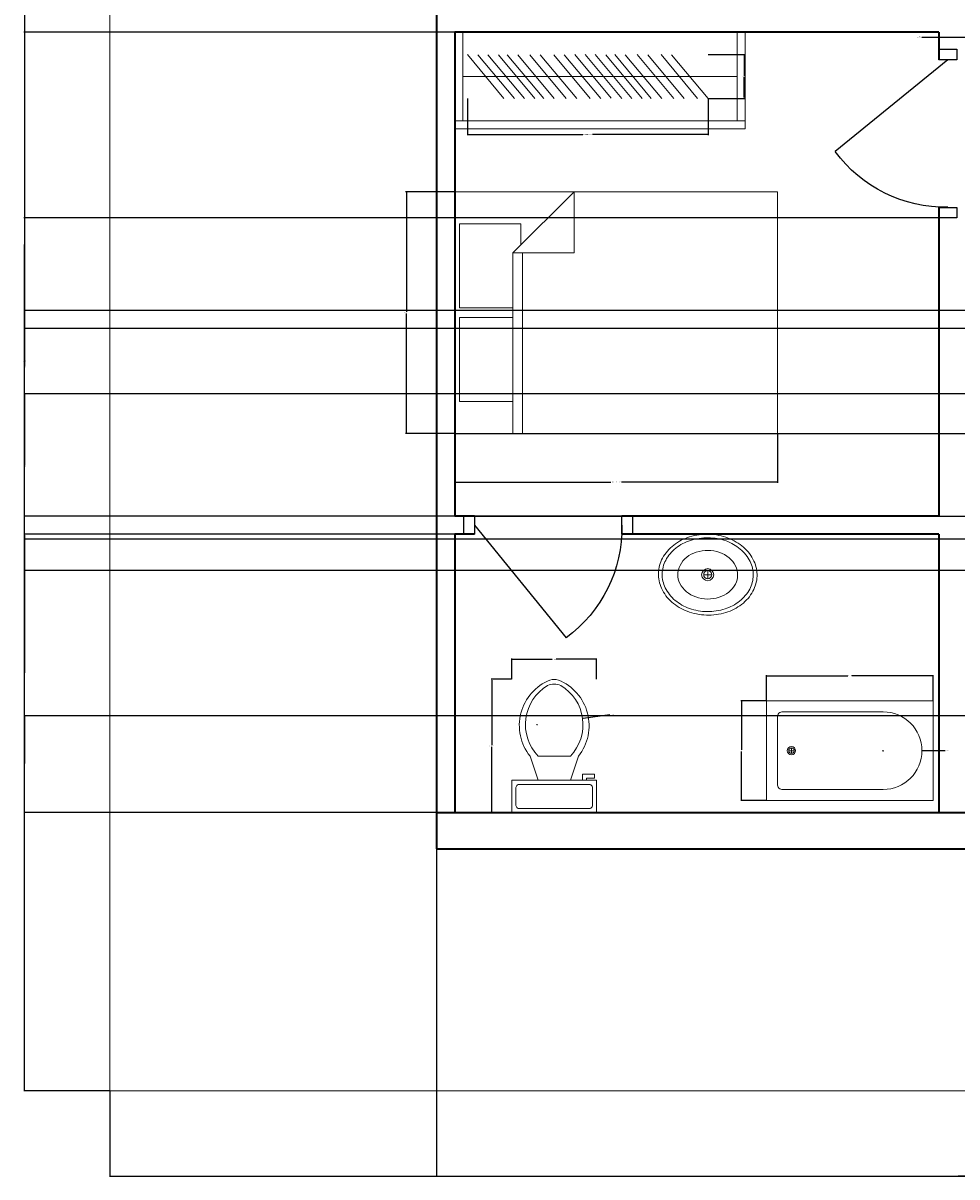
# Model space of a CAD drawing. Units: inches. Extents: x 109 to 572, y -157 to 568.
# Tile 1 of 5: x 109 to 341, y 105 to 391. Entities that reach past the tile are written whole.
import ezdxf

# ---------------------------------------------------------------- set-up
doc = ezdxf.new("R2010")
doc.units = ezdxf.units.IN
for name, color, linetype, lineweight in [('A-ANNO-DIMS', 2, 'Continuous', 18), ('A-FLOR-CASE', 32, 'Continuous', 18), ('A-FLOR-FIXT', 4, 'Continuous', 18), ('A-WALL', 7, 'Continuous', 35), ('C-PROP', 8, 'Continuous', 18), ('DOOR.', 240, 'Continuous', 25), ('FURNUTURE', 50, 'Continuous', 18)]:
    doc.layers.add(name, color=color, linetype=linetype, lineweight=lineweight)
doc.styles.get("Standard").update_dxf_attribs({"font": 'arial.ttf'})
doc.dimstyles.get("Standard").update_dxf_attribs({"dimtxt": 0.18, "dimasz": 0.18, "dimexe": 0.18, "dimexo": 0.0625, "dimgap": 0.09, "dimtad": 0, "dimtih": 1, "dimtoh": 1, "dimdec": 4, "dimzin": 0, "dimdsep": 46, "dimtxsty": 'Standard', "dimcen": 0.09, "dimadec": 0, "dimazin": 0, "dimtfac": 1, "dimtdec": 4, "dimtofl": 0, "dimtmove": 0, "dimatfit": 3, "dimfxl": 1, "dimtolj": 1, "dimtzin": 0, "dimarcsym": 0})

# ---------------------------------------------------------------- blocks, each defined once
blk = doc.blocks.new('Sink - Oval top')
for p, q in [((-1, 0), (1, 0)), ((0, 1), (0, -1))]:
    blk.add_line(p, q)
for points in [[(-12.23, 0.39, 0.117634), (-11.46, -3.36, 0.104469), (-8.88, -6.8, 0.090016), (-5.08, -9.07, 0.08192), (-0.32, -10.02, 0.08192), (4.49, -9.38, 0.090016), (8.42, -7.36, 0.104469), (11.22, -4.09, 0.117634), (12.23, -0.39, 0.117634), (11.46, 3.36, 0.104469), (8.88, 6.8, 0.090016), (5.08, 9.07, 0.08192), (0.32, 10.02, 0.08192), (-4.49, 9.38, 0.090016), (-8.42, 7.36, 0.104469), (-11.22, 4.09, 0.117634)], [(-11.29, 0.16, 0.118622), (-10.52, -3.25, 0.104678), (-8.07, -6.36, 0.089562), (-4.54, -8.37, 0.081185), (-0.13, -9.15, 0.081185), (4.3, -8.49, 0.089562), (7.89, -6.58, 0.104678), (10.42, -3.55, 0.118622), (11.29, -0.16, 0.118622), (10.52, 3.25, 0.104678), (8.07, 6.36, 0.089562), (4.54, 8.37, 0.081185), (0.13, 9.15, 0.081185), (-4.3, 8.49, 0.089562), (-7.89, 6.58, 0.104678), (-10.42, 3.55, 0.118622)], [(-7.42, 0.08, 0.118283), (-6.91, -2.17, 0.104607), (-5.29, -4.21, 0.089718), (-2.97, -5.53, 0.081436), (-0.07, -6.04, 0.081436), (2.84, -5.59, 0.089718), (5.2, -4.33, 0.104607), (6.86, -2.32, 0.118283), (7.42, -0.08, 0.118283), (6.91, 2.17, 0.104607), (5.29, 4.21, 0.089718), (2.97, 5.53, 0.081436), (0.07, 6.04, 0.081436), (-2.84, 5.59, 0.089718), (-5.2, 4.33, 0.104607), (-6.86, 2.32, 0.118283)]]:
    blk.add_lwpolyline(points, format="xyb", close=True)
for radius in [1.5, 1]:
    blk.add_circle((0, 0), radius)
blk = doc.blocks.new('Bath Tub - 26 x 60 in.')
for p, q in [((8, -18), (10, -18)), ((9, -17), (9, -19))]:
    blk.add_line(p, q)
blk.add_lwpolyline([(0, -36), (0, 0), (60, 0), (60, -36)], close=True)
for points in [[(6, -4), (42, -4)], [(4, -30), (4, -6)], [(42, -32), (6, -32)]]:
    blk.add_lwpolyline(points)
for radius in [1.5, 1]:
    blk.add_circle((9, -18), radius)
for centre, radius, start, end in [((5.75, -5.75), 1.77, 81.8699, 188.1301), ((42, -18), 14, 270, 90), ((5.75, -30.25), 1.77, 171.8699, 278.1301)]:
    blk.add_arc(centre, radius, start, end)
blk = doc.blocks.new('Bed - Queen')
for p, q in [((0, -80.00003), (0, 0)), ((0, 0), (59.99999, 0)), ((59.99999, 0), (59.99999, -80.00003)), ((7.99999, -1.2), (28.79998, -1.2)), ((7.99999, -14.4), (7.99999, -1.2)), ((28.79998, -1.2), (28.79998, -14.4)), ((31.19999, -1.2), (51.99999, -1.2)), ((31.19999, -14.4), (31.19999, -1.2)), ((51.99999, -1.2), (51.99999, -16.4)), ((0, -14.4), (44.8, -14.4)), ((44.8, -16.8), (0, -16.8)), ((59.99999, -29.6), (44.8, -14.4)), ((44.8, -14.4), (44.8, -29.6)), ((51.99999, -16.4), (46.79936, -16.4)), ((44.8, -29.6), (59.99999, -29.6)), ((59.99999, -80.00003), (0, -80.00003))]:
    blk.add_line(p, q)
blk = doc.blocks.new('Toilet - top')
for p, q in [((9.5, -6), (9.5, -2)), ((-10, -8.5), (-8, -8.5)), ((-10, -9.5), (-10, -8.5)), ((-8, -8.5), (-8, -8)), ((-7, -8), (-7, -9.5)), ((-4, -8), (-6, -14)), ((4, -8), (6, -14)), ((-7, -9.5), (-10, -9.5)), ((4, -14), (-4, -14))]:
    blk.add_line(p, q)
blk.add_lwpolyline([(10.5, -8), (10.5, 0), (-10.5, 0), (-10.5, -8)], close=True)
for points in [[(-9.5, -2), (-9.5, -6)], [(8.5, -1), (-8.5, -1)], [(-8.5, -7), (8.5, -7)]]:
    blk.add_lwpolyline(points)
for centre, radius, start, end in [((-8.62, -1.88), 0.884, 81.8699, 188.1301), ((8.62, -1.88), 0.884, 351.8699, 98.1301), ((-8.62, -6.12), 0.884, 171.8699, 278.1301), ((8.62, -6.12), 0.884, 261.8699, 8.1301), ((3.52, -21.58), 12.17, 141.4691, 247.9714), ((4.2, -21.82), 11.33, 136.3677, 238.9468), ((-3.52, -21.58), 12.17, 292.0284, 38.5307), ((-4.2, -21.82), 11.33, 301.053, 43.6321), ((0, -27.88), 4, 245.7318, 294.2682), ((0, -29), 4, 254.8605, 285.1395)]:
    blk.add_arc(centre, radius, start, end)
blk = doc.blocks.new('DOOR-SINGLE-36IN-JAMB')
blk.add_line((0, 0), (-27.91, 22.73))
for points in [[(-2.25, 36.57), (2.25, 36.57), (2.25, 39.21), (-2.25, 39.21)], [(-2.25, -2.64), (2.25, -2.64), (2.25, 0), (-2.25, 0)]]:
    blk.add_lwpolyline(points, close=True)
blk.add_arc((-0.58, 2.67), 33.9, 89.0125, 143.7179)
blk = doc.blocks.new('CLOSET-FRAME-RAIL-72IN')
for p, q in [((0, 0), (0, 24)), ((0, 24), (72, 24)), ((72, 24), (72, 0)), ((0, 22), (72, 22)), ((2, 0), (2, 22)), ((70, 22), (70, 0)), ((2, 11), (70, 11))]:
    blk.add_line(p, q)
blk = doc.blocks.new('CLOSET-HANGERS')
for p, q in [((0, 0), (-9.05, 10.83)), ((2.61, -0.01), (-6.44, 10.82)), ((5.08, -0.01), (-3.97, 10.82)), ((7.69, -0.01), (-1.36, 10.82)), ((9.9, -0.01), (0.85, 10.82)), ((12.51, -0.01), (3.46, 10.82)), ((15.48, -0.01), (6.43, 10.82)), ((18.09, -0.01), (9.04, 10.82)), ((21.4, -0.01), (12.35, 10.82)), ((24.01, -0.01), (14.96, 10.82)), ((26.62, 0.01), (17.57, 10.84)), ((29.23, 0), (20.18, 10.83)), ((31.7, 0), (22.65, 10.83)), ((34.31, -0.01), (25.26, 10.82)), ((36.52, 0), (27.47, 10.83)), ((39.13, -0.01), (30.08, 10.82)), ((42.1, 0), (33.05, 10.83)), ((44.71, -0.01), (35.66, 10.82)), ((48.01, 0), (38.97, 10.83)), ((50.63, -0.01), (41.58, 10.82))]:
    blk.add_line(p, q)
blk = doc.blocks.new('*D17')
at = {"layer": 'A-ANNO-DIMS', "color": 0, "lineweight": -2, "transparency": 16777216}
for p, q in [((216.02, 289.43), (216.02, 277.31)), ((296.02, 289.43), (296.02, 277.31)), ((216.2, 277.49), (254.72, 277.49)), ((295.84, 277.49), (257.32, 277.49))]:
    blk.add_line(p, q, dxfattribs=at)
at = {"layer": 'A-ANNO-DIMS', "color": 0, "transparency": 16777216}
for points in [[(216.2, 277.52), (216.2, 277.46), (216.02, 277.49)], [(295.84, 277.52), (295.84, 277.46), (296.02, 277.49)]]:
    blk.add_solid(points, dxfattribs=at)
at = {"layer": 'Defpoints', "color": 0, "transparency": 16777216}
for p in [(216.02, 289.49), (296.02, 289.49), (216.02, 277.49)]:
    blk.add_point(p, dxfattribs=at)
at = {"layer": 'A-ANNO-DIMS', "color": 0, "transparency": 16777216, "insert": (256.02, 277.49), "char_height": 0.18, "attachment_point": 5}
blk.add_mtext('\\A1;QUEEN BED 80 TYP.', dxfattribs=at)
blk = doc.blocks.new('*D18')
at = {"layer": 'A-ANNO-DIMS', "color": 0, "lineweight": -2, "transparency": 16777216}
for p, q in [((215.96, 349.49), (203.84, 349.49)), ((204.02, 349.31), (204.02, 319.67)), ((204.02, 289.67), (204.02, 319.31)), ((215.96, 289.49), (203.84, 289.49))]:
    blk.add_line(p, q, dxfattribs=at)
at = {"layer": 'A-ANNO-DIMS', "color": 0, "transparency": 16777216}
for points in [[(203.99, 349.31), (204.05, 349.31), (204.02, 349.49)], [(203.99, 289.67), (204.05, 289.67), (204.02, 289.49)]]:
    blk.add_solid(points, dxfattribs=at)
at = {"layer": 'Defpoints', "color": 0, "transparency": 16777216}
for p in [(204.02, 349.49), (216.02, 349.49), (216.02, 289.49)]:
    blk.add_point(p, dxfattribs=at)
at = {"layer": 'A-ANNO-DIMS', "color": 0, "transparency": 16777216, "insert": (204.02, 319.49), "char_height": 0.18, "attachment_point": 5}
blk.add_mtext('\\A1;60 TYP.', dxfattribs=at)
blk = doc.blocks.new('*D23')
at = {"layer": 'A-ANNO-DIMS', "color": 0, "lineweight": -2, "transparency": 16777216}
for p, q in [((230.11, 228.59), (225.04, 228.59)), ((225.22, 228.41), (225.22, 212.25)), ((225.22, 195.72), (225.22, 211.88)), ((230.11, 195.54), (225.04, 195.54))]:
    blk.add_line(p, q, dxfattribs=at)
at = {"layer": 'A-ANNO-DIMS', "color": 0, "transparency": 16777216}
for points in [[(225.19, 228.41), (225.25, 228.41), (225.22, 228.59)], [(225.19, 195.72), (225.25, 195.72), (225.22, 195.54)]]:
    blk.add_solid(points, dxfattribs=at)
at = {"layer": 'Defpoints', "color": 0, "transparency": 16777216}
for p in [(230.18, 228.59), (225.22, 195.54), (230.18, 195.54)]:
    blk.add_point(p, dxfattribs=at)
at = {"layer": 'A-ANNO-DIMS', "color": 0, "transparency": 16777216, "insert": (225.22, 212.06), "char_height": 0.18, "attachment_point": 5}
blk.add_mtext('\\A1;WC 33 TYP.', dxfattribs=at)
blk = doc.blocks.new('*D24')
at = {"layer": 'A-ANNO-DIMS', "color": 0, "lineweight": -2, "transparency": 16777216}
for p, q in [((230.18, 228.65), (230.18, 233.72)), ((230.36, 233.54), (240.15, 233.54)), ((251, 233.54), (241.2, 233.54)), ((251.18, 228.65), (251.18, 233.72))]:
    blk.add_line(p, q, dxfattribs=at)
at = {"layer": 'A-ANNO-DIMS', "color": 0, "transparency": 16777216}
for points in [[(230.36, 233.57), (230.36, 233.51), (230.18, 233.54)], [(251, 233.57), (251, 233.51), (251.18, 233.54)]]:
    blk.add_solid(points, dxfattribs=at)
at = {"layer": 'Defpoints', "color": 0, "transparency": 16777216}
for p in [(230.18, 233.54), (230.18, 228.59), (251.18, 228.59)]:
    blk.add_point(p, dxfattribs=at)
at = {"layer": 'A-ANNO-DIMS', "color": 0, "transparency": 16777216, "insert": (240.68, 233.54), "char_height": 0.18, "attachment_point": 5}
blk.add_mtext('\\A1;21 TYP.', dxfattribs=at)
blk = doc.blocks.new('*D27')
at = {"layer": 'A-ANNO-DIMS', "color": 0, "lineweight": -2, "transparency": 16777216}
for p, q in [((219.15, 372.56), (219.15, 363.49)), ((278.82, 372.56), (278.82, 363.49)), ((219.33, 363.67), (247.81, 363.67)), ((278.64, 363.67), (250.16, 363.67))]:
    blk.add_line(p, q, dxfattribs=at)
at = {"layer": 'A-ANNO-DIMS', "color": 0, "transparency": 16777216}
for points in [[(219.33, 363.7), (219.33, 363.64), (219.15, 363.67)], [(278.64, 363.7), (278.64, 363.64), (278.82, 363.67)]]:
    blk.add_solid(points, dxfattribs=at)
at = {"layer": 'Defpoints', "color": 0, "transparency": 16777216}
for p in [(219.15, 372.62), (278.82, 372.62), (278.82, 363.67)]:
    blk.add_point(p, dxfattribs=at)
at = {"layer": 'A-ANNO-DIMS', "color": 0, "transparency": 16777216, "insert": (248.99, 363.67), "char_height": 0.18, "attachment_point": 5}
blk.add_mtext('\\A1;HANGERS 60 TYP.', dxfattribs=at)
blk = doc.blocks.new('*D28')
at = {"layer": 'A-ANNO-DIMS', "color": 0, "lineweight": -2, "transparency": 16777216}
for p, q in [((278.88, 383.47), (287.95, 383.47)), ((287.77, 383.29), (287.77, 378.22)), ((287.77, 372.8), (287.77, 377.86)), ((278.88, 372.62), (287.95, 372.62))]:
    blk.add_line(p, q, dxfattribs=at)
at = {"layer": 'A-ANNO-DIMS', "color": 0, "transparency": 16777216}
for points in [[(287.74, 383.29), (287.8, 383.29), (287.77, 383.47)], [(287.74, 372.8), (287.8, 372.8), (287.77, 372.62)]]:
    blk.add_solid(points, dxfattribs=at)
at = {"layer": 'Defpoints', "color": 0, "transparency": 16777216}
for p in [(278.82, 383.47), (287.77, 383.47), (278.82, 372.62)]:
    blk.add_point(p, dxfattribs=at)
at = {"layer": 'A-ANNO-DIMS', "color": 0, "transparency": 16777216, "insert": (287.77, 378.04), "char_height": 0.18, "attachment_point": 5}
blk.add_mtext('\\A1;11 TYP.', dxfattribs=at)
blk = doc.blocks.new('*D37')
at = {"layer": 'A-ANNO-DIMS', "color": 0, "lineweight": -2, "transparency": 16777216}
for p, q in [((293.3, 223.34), (293.3, 229.65)), ((293.48, 229.47), (313.46, 229.47)), ((334.41, 229.47), (314.44, 229.47)), ((334.59, 223.34), (334.59, 229.65))]:
    blk.add_line(p, q, dxfattribs=at)
at = {"layer": 'A-ANNO-DIMS', "color": 0, "transparency": 16777216}
for points in [[(293.48, 229.5), (293.48, 229.44), (293.3, 229.47)], [(334.41, 229.5), (334.41, 229.44), (334.59, 229.47)]]:
    blk.add_solid(points, dxfattribs=at)
at = {"layer": 'Defpoints', "color": 0, "transparency": 16777216}
for p in [(334.59, 229.47), (293.3, 223.28), (334.59, 223.28)]:
    blk.add_point(p, dxfattribs=at)
at = {"layer": 'A-ANNO-DIMS', "color": 0, "transparency": 16777216, "insert": (313.95, 229.47), "char_height": 0.18, "attachment_point": 5}
blk.add_mtext('\\A1;TUB 41', dxfattribs=at)
blk = doc.blocks.new('*D38')
at = {"layer": 'A-ANNO-DIMS', "color": 0, "lineweight": -2, "transparency": 16777216}
for p, q in [((293.24, 223.28), (286.93, 223.28)), ((287.11, 223.1), (287.11, 211.07)), ((287.11, 198.69), (287.11, 210.71)), ((293.24, 198.51), (286.93, 198.51))]:
    blk.add_line(p, q, dxfattribs=at)
at = {"layer": 'A-ANNO-DIMS', "color": 0, "transparency": 16777216}
for points in [[(287.08, 223.1), (287.14, 223.1), (287.11, 223.28)], [(287.08, 198.69), (287.14, 198.69), (287.11, 198.51)]]:
    blk.add_solid(points, dxfattribs=at)
at = {"layer": 'Defpoints', "color": 0, "transparency": 16777216}
for p in [(287.11, 223.28), (293.3, 223.28), (293.3, 198.51)]:
    blk.add_point(p, dxfattribs=at)
at = {"layer": 'A-ANNO-DIMS', "color": 0, "transparency": 16777216, "insert": (287.11, 210.89), "char_height": 0.18, "attachment_point": 5}
blk.add_mtext('\\A1;25', dxfattribs=at)
blk = doc.blocks.new('*D39')
at = {"layer": 'A-ANNO-DIMS', "color": 0, "lineweight": -2, "transparency": 16777216}
for p, q in [((130.52, 126.48), (130.52, 105.21)), ((550.52, 126.48), (550.52, 105.21)), ((130.7, 105.39), (340.23, 105.39)), ((550.34, 105.39), (340.81, 105.39))]:
    blk.add_line(p, q, dxfattribs=at)
at = {"layer": 'A-ANNO-DIMS', "color": 0, "transparency": 16777216}
for points in [[(130.7, 105.42), (130.7, 105.36), (130.52, 105.39)], [(550.34, 105.42), (550.34, 105.36), (550.52, 105.39)]]:
    blk.add_solid(points, dxfattribs=at)
at = {"layer": 'Defpoints', "color": 0, "transparency": 16777216}
for p in [(130.52, 126.54), (550.52, 126.54), (550.52, 105.39)]:
    blk.add_point(p, dxfattribs=at)
at = {"layer": 'A-ANNO-DIMS', "color": 0, "transparency": 16777216, "insert": (340.52, 105.39), "char_height": 0.18, "attachment_point": 5}
blk.add_mtext('\\A1;420', dxfattribs=at)
blk = doc.blocks.new('*D40')
at = {"layer": 'A-ANNO-DIMS', "color": 0, "lineweight": -2, "transparency": 16777216}
for p, q in [((130.46, 546.54), (109.19, 546.54)), ((109.37, 546.36), (109.37, 336.72)), ((109.37, 126.72), (109.37, 336.36)), ((130.46, 126.54), (109.19, 126.54))]:
    blk.add_line(p, q, dxfattribs=at)
at = {"layer": 'A-ANNO-DIMS', "color": 0, "transparency": 16777216}
for points in [[(109.34, 546.36), (109.4, 546.36), (109.37, 546.54)], [(109.34, 126.72), (109.4, 126.72), (109.37, 126.54)]]:
    blk.add_solid(points, dxfattribs=at)
at = {"layer": 'Defpoints', "color": 0, "transparency": 16777216}
for p in [(109.37, 546.54), (130.52, 546.54), (130.52, 126.54)]:
    blk.add_point(p, dxfattribs=at)
at = {"layer": 'A-ANNO-DIMS', "color": 0, "transparency": 16777216, "insert": (109.37, 336.54), "char_height": 0.18, "attachment_point": 5}
blk.add_mtext('\\A1;420', dxfattribs=at)
blk = doc.blocks.new('*D43')
at = {"layer": 'A-ANNO-DIMS', "color": 0, "lineweight": -2, "transparency": 16777216}
for p, q in [((211.52, 186.48), (211.52, 105.21)), ((526.52, 186.48), (526.52, 105.21)), ((211.7, 105.39), (368.73, 105.39)), ((526.34, 105.39), (369.31, 105.39))]:
    blk.add_line(p, q, dxfattribs=at)
at = {"layer": 'A-ANNO-DIMS', "color": 0, "transparency": 16777216}
for points in [[(211.7, 105.42), (211.7, 105.36), (211.52, 105.39)], [(526.34, 105.42), (526.34, 105.36), (526.52, 105.39)]]:
    blk.add_solid(points, dxfattribs=at)
at = {"layer": 'Defpoints', "color": 0, "transparency": 16777216}
for p in [(211.52, 186.54), (526.52, 186.54), (526.52, 105.39)]:
    blk.add_point(p, dxfattribs=at)
at = {"layer": 'A-ANNO-DIMS', "color": 0, "transparency": 16777216, "insert": (369.02, 105.39), "char_height": 0.18, "attachment_point": 5}
blk.add_mtext('\\A1;315', dxfattribs=at)
blk = doc.blocks.new('*D48')
at = {"layer": 'A-ANNO-DIMS', "color": 0, "lineweight": -2, "transparency": 16777216}
for p, q in [((215.96, 264.54), (109.19, 264.54)), ((109.37, 264.36), (109.37, 230.22)), ((109.37, 195.72), (109.37, 229.86)), ((215.96, 195.54), (109.19, 195.54))]:
    blk.add_line(p, q, dxfattribs=at)
at = {"layer": 'A-ANNO-DIMS', "color": 0, "transparency": 16777216}
for points in [[(109.34, 264.36), (109.4, 264.36), (109.37, 264.54)], [(109.34, 195.72), (109.4, 195.72), (109.37, 195.54)]]:
    blk.add_solid(points, dxfattribs=at)
at = {"layer": 'Defpoints', "color": 0, "transparency": 16777216}
for p in [(109.37, 264.54), (216.02, 264.54), (216.02, 195.54)]:
    blk.add_point(p, dxfattribs=at)
at = {"layer": 'A-ANNO-DIMS', "color": 0, "transparency": 16777216, "insert": (109.37, 230.04), "char_height": 0.18, "attachment_point": 5}
blk.add_mtext('\\A1;69', dxfattribs=at)
blk = doc.blocks.new('*D49')
at = {"layer": 'A-ANNO-DIMS', "color": 0, "lineweight": -2, "transparency": 16777216}
for p, q in [((215.96, 389.04), (109.19, 389.04)), ((109.37, 388.86), (109.37, 329.22)), ((109.37, 269.22), (109.37, 328.86)), ((215.96, 269.04), (109.19, 269.04))]:
    blk.add_line(p, q, dxfattribs=at)
at = {"layer": 'A-ANNO-DIMS', "color": 0, "transparency": 16777216}
for points in [[(109.34, 388.86), (109.4, 388.86), (109.37, 389.04)], [(109.34, 269.22), (109.4, 269.22), (109.37, 269.04)]]:
    blk.add_solid(points, dxfattribs=at)
at = {"layer": 'Defpoints', "color": 0, "transparency": 16777216}
for p in [(109.37, 389.04), (216.02, 389.04), (216.02, 269.04)]:
    blk.add_point(p, dxfattribs=at)
at = {"layer": 'A-ANNO-DIMS', "color": 0, "transparency": 16777216, "insert": (109.37, 329.04), "char_height": 0.18, "attachment_point": 5}
blk.add_mtext('\\A1;120', dxfattribs=at)
blk = doc.blocks.new('*D55')
at = {"layer": 'A-ANNO-DIMS', "color": 0, "lineweight": -2, "transparency": 16777216}
for p, q in [((493.46, 299.4), (109.19, 299.4)), ((109.37, 299.22), (109.37, 281.56)), ((109.37, 263.53), (109.37, 281.2)), ((493.46, 263.35), (109.19, 263.35))]:
    blk.add_line(p, q, dxfattribs=at)
at = {"layer": 'A-ANNO-DIMS', "color": 0, "transparency": 16777216}
for points in [[(109.34, 299.22), (109.4, 299.22), (109.37, 299.4)], [(109.34, 263.53), (109.4, 263.53), (109.37, 263.35)]]:
    blk.add_solid(points, dxfattribs=at)
at = {"layer": 'Defpoints', "color": 0, "transparency": 16777216}
for p in [(109.37, 299.4), (493.52, 299.4), (493.52, 263.35)]:
    blk.add_point(p, dxfattribs=at)
at = {"layer": 'A-ANNO-DIMS', "color": 0, "transparency": 16777216, "insert": (109.37, 281.38), "char_height": 0.18, "attachment_point": 5}
blk.add_mtext('\\A1;36.05', dxfattribs=at)
blk = doc.blocks.new('*D56')
at = {"layer": 'A-ANNO-DIMS', "color": 0, "lineweight": -2, "transparency": 16777216}
for p, q in [((493.46, 255.54), (109.19, 255.54)), ((109.37, 255.36), (109.37, 237.72)), ((109.37, 219.72), (109.37, 237.36)), ((493.46, 219.54), (109.19, 219.54))]:
    blk.add_line(p, q, dxfattribs=at)
at = {"layer": 'A-ANNO-DIMS', "color": 0, "transparency": 16777216}
for points in [[(109.34, 255.36), (109.4, 255.36), (109.37, 255.54)], [(109.34, 219.72), (109.4, 219.72), (109.37, 219.54)]]:
    blk.add_solid(points, dxfattribs=at)
at = {"layer": 'Defpoints', "color": 0, "transparency": 16777216}
for p in [(493.52, 255.54), (109.37, 219.54), (493.52, 219.54)]:
    blk.add_point(p, dxfattribs=at)
at = {"layer": 'A-ANNO-DIMS', "color": 0, "transparency": 16777216, "insert": (109.37, 237.54), "char_height": 0.18, "attachment_point": 5}
blk.add_mtext('\\A1;36', dxfattribs=at)
blk = doc.blocks.new('*D58')
at = {"layer": 'A-ANNO-DIMS', "color": 0, "lineweight": -2, "transparency": 16777216}
for p, q in [((335.96, 342.97), (109.19, 342.97)), ((109.37, 342.79), (109.37, 306.19)), ((109.37, 269.22), (109.37, 305.82)), ((335.96, 269.04), (109.19, 269.04))]:
    blk.add_line(p, q, dxfattribs=at)
at = {"layer": 'A-ANNO-DIMS', "color": 0, "transparency": 16777216}
for points in [[(109.34, 342.79), (109.4, 342.79), (109.37, 342.97)], [(109.34, 269.22), (109.4, 269.22), (109.37, 269.04)]]:
    blk.add_solid(points, dxfattribs=at)
at = {"layer": 'Defpoints', "color": 0, "transparency": 16777216}
for p in [(109.37, 342.97), (336.02, 342.97), (336.02, 269.04)]:
    blk.add_point(p, dxfattribs=at)
at = {"layer": 'A-ANNO-DIMS', "color": 0, "transparency": 16777216, "insert": (109.37, 306), "char_height": 0.18, "attachment_point": 5}
blk.add_mtext('\\A1;73.93', dxfattribs=at)
blk = doc.blocks.new('*D63')
at = {"layer": 'A-ANNO-DIMS', "color": 0, "lineweight": -2, "transparency": 16777216}
for p, q in [((457.46, 320.04), (109.19, 320.04)), ((109.37, 319.86), (109.37, 317.97)), ((109.37, 315.72), (109.37, 317.61)), ((457.46, 315.54), (109.19, 315.54))]:
    blk.add_line(p, q, dxfattribs=at)
at = {"layer": 'A-ANNO-DIMS', "color": 0, "transparency": 16777216}
for points in [[(109.34, 319.86), (109.4, 319.86), (109.37, 320.04)], [(109.34, 315.72), (109.4, 315.72), (109.37, 315.54)]]:
    blk.add_solid(points, dxfattribs=at)
at = {"layer": 'Defpoints', "color": 0, "transparency": 16777216}
for p in [(109.37, 320.04), (457.52, 320.04), (457.52, 315.54)]:
    blk.add_point(p, dxfattribs=at)
at = {"layer": 'A-ANNO-DIMS', "color": 0, "transparency": 16777216, "insert": (109.37, 317.79), "char_height": 0.18, "attachment_point": 5}
blk.add_mtext('\\A1;4.5', dxfattribs=at)
blk = doc.blocks.new('*D67')
at = {"layer": 'A-ANNO-DIMS', "color": 0, "lineweight": -2, "transparency": 16777216}
for p, q in [((457.46, 219.54), (109.19, 219.54)), ((109.37, 219.36), (109.37, 207.72)), ((109.37, 195.72), (109.37, 207.36)), ((457.46, 195.54), (109.19, 195.54))]:
    blk.add_line(p, q, dxfattribs=at)
at = {"layer": 'A-ANNO-DIMS', "color": 0, "transparency": 16777216}
for points in [[(109.34, 219.36), (109.4, 219.36), (109.37, 219.54)], [(109.34, 195.72), (109.4, 195.72), (109.37, 195.54)]]:
    blk.add_solid(points, dxfattribs=at)
at = {"layer": 'Defpoints', "color": 0, "transparency": 16777216}
for p in [(457.52, 219.54), (109.37, 195.54), (457.52, 195.54)]:
    blk.add_point(p, dxfattribs=at)
at = {"layer": 'A-ANNO-DIMS', "color": 0, "transparency": 16777216, "insert": (109.37, 207.54), "char_height": 0.18, "attachment_point": 5}
blk.add_mtext('\\A1;24', dxfattribs=at)
blk = doc.blocks.new('*D69')
at = {"layer": 'A-ANNO-DIMS', "color": 0, "lineweight": -2, "transparency": 16777216}
for p, q in [((216.08, 289.49), (571.85, 289.49)), ((571.67, 289.31), (571.67, 279.45)), ((571.67, 269.22), (571.67, 279.08)), ((216.08, 269.04), (571.85, 269.04))]:
    blk.add_line(p, q, dxfattribs=at)
at = {"layer": 'A-ANNO-DIMS', "color": 0, "transparency": 16777216}
for points in [[(571.64, 289.31), (571.7, 289.31), (571.67, 289.49)], [(571.64, 269.22), (571.7, 269.22), (571.67, 269.04)]]:
    blk.add_solid(points, dxfattribs=at)
at = {"layer": 'Defpoints', "color": 0, "transparency": 16777216}
for p in [(216.02, 289.49), (571.67, 289.49), (216.02, 269.04)]:
    blk.add_point(p, dxfattribs=at)
at = {"layer": 'A-ANNO-DIMS', "color": 0, "transparency": 16777216, "insert": (571.67, 279.26), "char_height": 0.18, "attachment_point": 5}
blk.add_mtext('\\A1;20.45', dxfattribs=at)
blk = doc.blocks.new('*D70')
at = {"layer": 'A-ANNO-DIMS', "color": 0, "lineweight": -2, "transparency": 16777216}
for p, q in [((517.46, 315.54), (109.19, 315.54)), ((109.37, 315.36), (109.37, 307.65)), ((109.37, 299.58), (109.37, 307.29)), ((517.46, 299.4), (109.19, 299.4))]:
    blk.add_line(p, q, dxfattribs=at)
at = {"layer": 'A-ANNO-DIMS', "color": 0, "transparency": 16777216}
for points in [[(109.34, 315.36), (109.4, 315.36), (109.37, 315.54)], [(109.34, 299.58), (109.4, 299.58), (109.37, 299.4)]]:
    blk.add_solid(points, dxfattribs=at)
at = {"layer": 'Defpoints', "color": 0, "transparency": 16777216}
for p in [(517.52, 315.54), (109.37, 299.4), (517.52, 299.4)]:
    blk.add_point(p, dxfattribs=at)
at = {"layer": 'A-ANNO-DIMS', "color": 0, "transparency": 16777216, "insert": (109.37, 307.47), "char_height": 0.18, "attachment_point": 5}
blk.add_mtext('\\A1;16.136', dxfattribs=at)
blk = doc.blocks.new('*D74')
at = {"layer": 'A-ANNO-DIMS', "color": 0, "lineweight": -2, "transparency": 16777216}
for p, q in [((331.8, 387.8), (374.88, 387.8)), ((447.07, 387.8), (447.25, 387.8)), ((447.16, 387.71), (447.16, 387.89))]:
    blk.add_line(p, q, dxfattribs=at)
at = {"layer": 'A-ANNO-DIMS', "color": 0, "transparency": 16777216}
blk.add_solid([(374.88, 387.83), (374.88, 387.77), (375.06, 387.8)], dxfattribs=at)
at = {"layer": 'Defpoints', "color": 0, "transparency": 16777216}
for p in [(375.06, 387.8), (447.16, 387.8)]:
    blk.add_point(p, dxfattribs=at)
at = {"layer": 'A-ANNO-DIMS', "color": 0, "transparency": 16777216, "insert": (331.21, 387.8), "char_height": 0.18, "attachment_point": 5}
blk.add_mtext('\\A1;2X R72.1', dxfattribs=at)
blk = doc.blocks.new('*D76')
at = {"layer": 'A-ANNO-DIMS', "color": 0, "lineweight": -2, "transparency": 16777216}
for p, q in [((236.48, 217.27), (236.48, 217.45)), ((254.44, 219.77), (247.88, 218.89)), ((236.39, 217.36), (236.57, 217.36))]:
    blk.add_line(p, q, dxfattribs=at)
at = {"layer": 'A-ANNO-DIMS', "color": 0, "transparency": 16777216}
blk.add_solid([(247.88, 218.92), (247.89, 218.86), (247.7, 218.87)], dxfattribs=at)
at = {"layer": 'Defpoints', "color": 0, "transparency": 16777216}
for p in [(247.7, 218.87), (236.48, 217.36)]:
    blk.add_point(p, dxfattribs=at)
at = {"layer": 'A-ANNO-DIMS', "color": 0, "transparency": 16777216, "insert": (255.12, 219.77), "char_height": 0.18, "attachment_point": 5}
blk.add_mtext('\\A1;4X R11.33', dxfattribs=at)
blk = doc.blocks.new('*D78')
at = {"layer": 'A-ANNO-DIMS', "color": 0, "lineweight": -2, "transparency": 16777216}
for p, q in [((322.11, 210.89), (322.29, 210.89)), ((322.2, 210.8), (322.2, 210.98)), ((337.62, 210.89), (332.02, 210.89))]:
    blk.add_line(p, q, dxfattribs=at)
at = {"layer": 'A-ANNO-DIMS', "color": 0, "transparency": 16777216}
blk.add_solid([(332.02, 210.92), (332.02, 210.86), (331.84, 210.89)], dxfattribs=at)
at = {"layer": 'Defpoints', "color": 0, "transparency": 16777216}
for p in [(322.2, 210.89), (331.84, 210.89)]:
    blk.add_point(p, dxfattribs=at)
at = {"layer": 'A-ANNO-DIMS', "color": 0, "transparency": 16777216, "insert": (338.1, 210.89), "char_height": 0.18, "attachment_point": 5}
blk.add_mtext('\\A1;R9.634', dxfattribs=at)

msp = doc.modelspace()

# ---------------------------------------------------------------- linework, layer by layer
at = {"layer": 'A-WALL'}
for p, q in [((211.5195, 513.5398), (211.5195, 195.5398)), ((336.0195, 389.0398), (216.0195, 389.0398)), ((216.0195, 389.0398), (216.0195, 269.0398)), ((336.0195, 389.0398), (336.0195, 382.1753)), ((336.0195, 345.6414), (336.0195, 269.0398)), ((220.8949, 269.0398), (216.0195, 269.0398)), ((336.0195, 269.0398), (257.4647, 269.0398)), ((216.0195, 264.5398), (216.0195, 195.5398)), ((220.8949, 264.5398), (216.0195, 264.5398)), ((336.0195, 264.5398), (257.4288, 264.5398)), ((336.0195, 264.5398), (336.0195, 195.5398)), ((211.5195, 195.5398), (517.5195, 195.5398)), ((211.5195, 195.5398), (211.5195, 186.5398)), ((211.5195, 186.5398), (526.5195, 186.5398))]:
    msp.add_line(p, q, dxfattribs=at)
at = {"layer": 'C-PROP'}
for p, q in [((130.5195, 546.5398), (130.5195, 126.5398)), ((130.5195, 126.5398), (550.5195, 126.5398))]:
    msp.add_line(p, q, dxfattribs=at)

# ---------------------------------------------------------------- block references
at = {"layer": 'A-FLOR-CASE', "rotation": 180}
msp.add_blockref('CLOSET-FRAME-RAIL-72IN', (288.0195, 389.0398), dxfattribs=at)
at = {"layer": 'A-FLOR-CASE'}
msp.add_blockref('CLOSET-HANGERS', (228.1956, 372.6308), dxfattribs=at)
at = {"layer": 'A-FLOR-FIXT'}
msp.add_blockref('Sink - Oval top', (278.7316, 254.5239), dxfattribs=at)
at = {"layer": 'A-FLOR-FIXT', "rotation": 180}
msp.add_blockref('Toilet - top', (240.6752, 195.5398), dxfattribs=at)
at = {"layer": 'A-FLOR-FIXT', "xscale": 0.6881205280154126, "yscale": 0.6881205280154126, "zscale": 0.6881205280154126}
msp.add_blockref('Bath Tub - 26 x 60 in.', (293.3019, 223.2784), dxfattribs=at)
at = {"layer": 'DOOR.', "extrusion": (0, 0, -1), "zscale": -1}
for p, rotation in [((-338.2695, 382.1753), 180), ((-220.8949, 266.7898), 89.99999999999979)]:
    msp.add_blockref('DOOR-SINGLE-36IN-JAMB', p, dxfattribs=dict(at, rotation=rotation))
at = {"layer": 'FURNUTURE', "rotation": 90}
msp.add_blockref('Bed - Queen', (216.0195, 289.4894), dxfattribs=at)

# ---------------------------------------------------------------- dimensions: what is measured, and where the dimension line sits
at = {"layer": 'A-ANNO-DIMS'}
for base, p1, p2, override, picture, middle in [((109.3695, 546.5398), (130.5195, 126.5398), (130.5195, 546.5398), {"dimdec": 0, "dimlfac": 1, "dimrnd": 0, "dimzin": 0, "dimdsep": 46, "dimlunit": 2}, '*D40', (109.3695, 336.5398)), ((109.3695, 389.0398), (216.0195, 269.0398), (216.0195, 389.0398), {"dimdec": 0, "dimlfac": 1, "dimrnd": 0, "dimzin": 0, "dimdsep": 46, "dimlunit": 2}, '*D49', (109.3695, 329.0398)), ((109.3695, 342.9664), (336.0195, 269.0398), (336.0195, 342.9664), {"dimdec": 2, "dimlfac": 1, "dimrnd": 0, "dimzin": 0, "dimdsep": 46, "dimlunit": 2}, '*D58', (109.3695, 306.0031)), ((109.3695, 320.0398), (457.5195, 315.5398), (457.5195, 320.0398), {"dimdec": 1, "dimlfac": 1, "dimrnd": 0, "dimzin": 0, "dimdsep": 46, "dimlunit": 2}, '*D63', (109.3695, 317.7898)), ((109.3695, 299.4036), (517.5195, 315.5398), (517.5195, 299.4036), {"dimdec": 3, "dimlfac": 1, "dimrnd": 0, "dimzin": 0, "dimdsep": 46, "dimlunit": 2}, '*D70', (109.3695, 307.4717)), ((109.3695, 299.4036), (493.5195, 263.3515), (493.5195, 299.4036), {"dimdec": 2, "dimlfac": 1, "dimrnd": 0, "dimzin": 0, "dimdsep": 46, "dimlunit": 2}, '*D55', (109.3695, 281.3775)), ((571.6695, 289.4894), (216.0195, 269.0398), (216.0195, 289.4894), {"dimdec": 2, "dimlfac": 1, "dimrnd": 0, "dimzin": 0, "dimdsep": 46, "dimlunit": 2}, '*D69', (571.6695, 279.2646)), ((109.3695, 264.5398), (216.0195, 195.5398), (216.0195, 264.5398), {"dimdec": 0, "dimlfac": 1, "dimrnd": 0, "dimzin": 0, "dimdsep": 46, "dimlunit": 2}, '*D48', (109.3695, 230.0398)), ((109.3695, 219.5398), (493.5195, 255.5398), (493.5195, 219.5398), {"dimdec": 0, "dimlfac": 1, "dimrnd": 0, "dimzin": 0, "dimdsep": 46, "dimlunit": 2}, '*D56', (109.3695, 237.5398)), ((287.1088, 223.2784), (293.3019, 198.506), (293.3019, 223.2784), {"dimdec": 0, "dimlfac": 1, "dimrnd": 0, "dimzin": 0, "dimdsep": 46, "dimlunit": 2}, '*D38', (287.1088, 210.8922)), ((109.3695, 195.5398), (457.5195, 219.5398), (457.5195, 195.5398), {"dimdec": 0, "dimlfac": 1, "dimrnd": 0, "dimzin": 0, "dimdsep": 46, "dimlunit": 2}, '*D67', (109.3695, 207.5398))]:
    dim = msp.add_linear_dim(base=base, p1=p1, p2=p2, angle=90, dimstyle='Standard', override=override, dxfattribs=at)
    dim.commit()
    dim.dimension.update_dxf_attribs({"geometry": picture, "text_midpoint": middle})
for center, mpoint, text, override, picture, middle in [((447.1629, 387.7979), (375.058, 387.798), '2X <>', {"dimdec": 1, "dimlfac": 1, "dimrnd": 0, "dimzin": 0, "dimdsep": 46, "dimlunit": 2}, '*D74', (331.7951, 387.7981)), ((236.4752, 217.3572), (247.7033, 218.867), '4X <>', {"dimdec": 2, "dimlfac": 1, "dimrnd": 0, "dimzin": 0, "dimdsep": 46, "dimlunit": 2}, '*D76', (254.4402, 219.773))]:
    dim = msp.add_radius_dim(center=center, mpoint=mpoint, text=text, dimstyle='Standard', override=override, dxfattribs=at)
    dim.commit()
    dim.dimension.update_dxf_attribs({"geometry": picture, "text_midpoint": middle, "dimtype": 164})
for base, p1, p2, angle, text, picture, middle in [((287.772, 383.466), (278.8212, 372.6193), (278.8212, 383.466), 90, '<> TYP.', '*D28', (287.772, 378.0427)), ((204.0195, 349.4894), (216.0195, 289.4894), (216.0195, 349.4894), 90, '<> TYP.', '*D18', (204.0195, 319.4894)), ((216.0195, 277.4894), (296.0196, 289.4894), (216.0195, 289.4894), 180, 'QUEEN BED <> TYP.', '*D17', (256.0196, 277.4894)), ((230.1752, 233.543), (251.1752, 228.586), (230.1752, 228.586), 180, '<> TYP.', '*D24', (240.6752, 233.543)), ((225.2182, 195.5398), (230.1752, 228.586), (230.1752, 195.5398), 270, 'WC <> TYP.', '*D23', (225.2182, 212.0629))]:
    dim = msp.add_linear_dim(base=base, p1=p1, p2=p2, angle=angle, text=text, dimstyle='Standard', override={"dimdec": 0, "dimlfac": 1, "dimrnd": 0, "dimzin": 0, "dimdsep": 46, "dimlunit": 2}, dxfattribs=at)
    dim.commit()
    dim.dimension.update_dxf_attribs({"geometry": picture, "text_midpoint": middle})
for base, p1, p2, text, picture, middle in [((278.8212, 363.6684), (219.1489, 372.6193), (278.8212, 372.6193), 'HANGERS <> TYP.', '*D27', (248.985, 363.6684)), ((334.5891, 229.4714), (293.3019, 223.2784), (334.5891, 223.2784), 'TUB <>', '*D37', (313.9455, 229.4714))]:
    dim = msp.add_linear_dim(base=base, p1=p1, p2=p2, text=text, dimstyle='Standard', override={"dimdec": 0, "dimlfac": 1, "dimrnd": 0, "dimzin": 0, "dimdsep": 46, "dimlunit": 2}, dxfattribs=at)
    dim.commit()
    dim.dimension.update_dxf_attribs({"geometry": picture, "text_midpoint": middle})
dim = msp.add_radius_dim(center=(322.203, 210.8922), mpoint=(331.8366, 210.892), dimstyle='Standard', override={"dimdec": 3, "dimlfac": 1, "dimrnd": 0, "dimzin": 0, "dimdsep": 46, "dimlunit": 2}, dxfattribs=at)
dim.commit()
dim.dimension.update_dxf_attribs({"geometry": '*D78', "text_midpoint": (337.6169, 210.8919), "dimtype": 164})
for base, p1, p2, picture, middle in [((526.5195, 105.3898), (211.5195, 186.5398), (526.5195, 186.5398), '*D43', (369.0195, 105.3898)), ((550.5195, 105.3898), (130.5195, 126.5398), (550.5195, 126.5398), '*D39', (340.5195, 105.3898))]:
    dim = msp.add_linear_dim(base=base, p1=p1, p2=p2, dimstyle='Standard', override={"dimdec": 0, "dimlfac": 1, "dimrnd": 0, "dimzin": 0, "dimdsep": 46, "dimlunit": 2}, dxfattribs=at)
    dim.commit()
    dim.dimension.update_dxf_attribs({"geometry": picture, "text_midpoint": middle})

doc.saveas('drawing.dxf')
